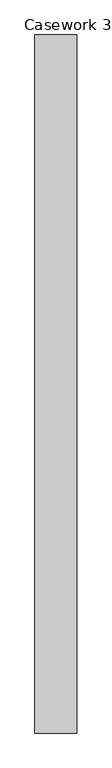
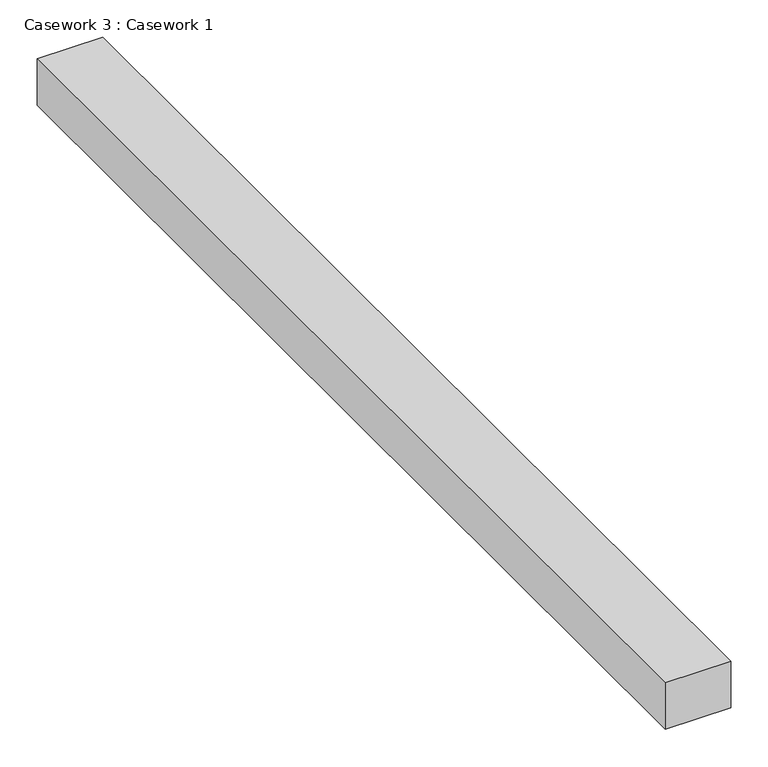
"""IFC4 building model written with IfcOpenShell, lengths in millimetres: furniture geometry, Casework 3 : Casework 1."""

from ifc_helpers import new_model, si_unit, frame, origin, place, context, project, spatial, polyline, outline, extrude, source, transform, mapped, element, save


def casework_3_casework_1_f196c302(model_context):
    return source(origin(), model_context, "Body", "SweptSolid", [
        extrude(outline(polyline([(9052.9559589, 14787.9496924), (9052.9559589, 13098.8496924), (8951.3559589, 13098.8496924), (8951.3559589, 14787.9496924), (9052.9559589, 14787.9496924)])), frame((0.0, 0.0, 3581.4), z_axis=(0.0, 0.0, 1.0), x_axis=(1.0, 0.0, 0.0)), (0.0, 0.0, 1.0), 76.2),
    ])


if __name__ == "__main__":
    model = new_model("IFC4")
    model_context = context("Model", 3, world=origin())
    ifc_project = project(units=[si_unit("LENGTHUNIT", "METRE", prefix="MILLI")], contexts=[model_context])
    site = spatial("IfcSite", under=ifc_project)
    building = spatial("IfcBuilding", under=site)
    placement = place(None, origin())
    casework_3_casework_1_shape = casework_3_casework_1_f196c302(model_context)
    element("IfcFurniture", 1, ObjectType="Casework 3 : Casework 1", at=placement, inside=building, context=model_context, shape_type="MappedRepresentation", body=[
        mapped(casework_3_casework_1_shape, transform((0.0, 0.0, 0.0), x_axis=(1.0, 0.0, 0.0), y_axis=(0.0, 1.0, 0.0), z_axis=(0.0, 0.0, 1.0))),
    ])
    save(model, "model.ifc")

# Revit data of these elements
# Element 1 (IfcFurniture, "Casework 3 : Casework 1")
#   Materials on its faces: "Clad - White"
# Materials
#   "Clad - White": class "Wood", colour RGB 242 242 238, transparency 0, Cost = 0
